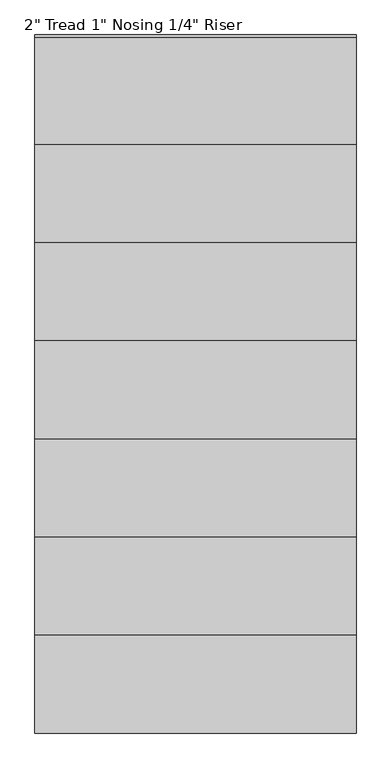
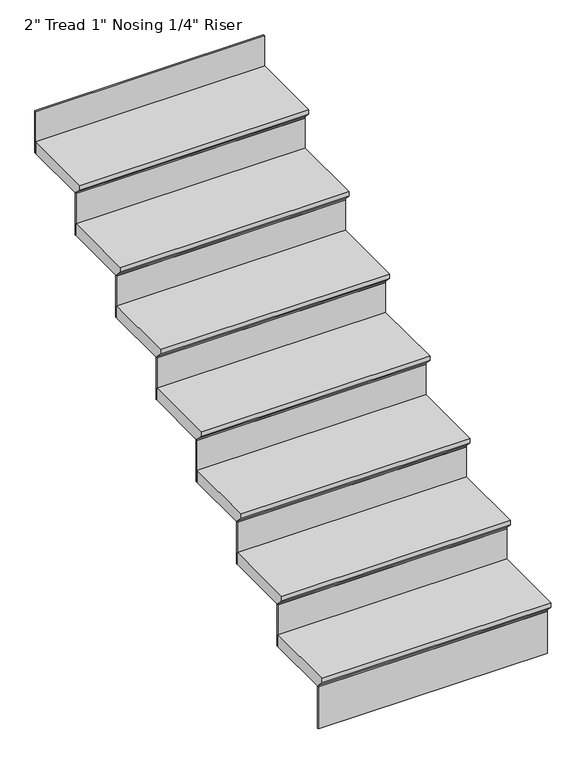
"""IFC4 building model written with IfcOpenShell, lengths in millimetres: stair flight geometry."""

from ifc_helpers import new_model, si_unit, frame, origin, place, context, project, spatial, polyline, outline, extrude, source, transform, mapped, element, save


def stair_flight_4d250dde(model_context):
    return source(origin(), model_context, "Body", "SweptSolid", [
        extrude(outline(polyline([(-3538.5064015, 5765.8), (-3233.7064015, 5765.8), (-3233.7064015, 5715.0), (-3513.1064015, 5715.0), (-3513.1064015, 5721.35), (-3538.5064015, 5746.75), (-3538.5064015, 5765.8)])), frame((-4591.1993763, 0.0, 0.0), z_axis=(1.0, 0.0, 0.0), x_axis=(0.0, 1.0, 0.0)), (0.0, 0.0, 1.0), 914.4),
        extrude(outline(polyline([(-3676.7993763, -3506.7564015), (-3676.7993763, -3513.1064015), (-4591.1993763, -3513.1064015), (-4591.1993763, -3506.7564015), (-3676.7993763, -3506.7564015)])), frame((0.0, 0.0, 5537.2), z_axis=(0.0, 0.0, 1.0), x_axis=(1.0, 0.0, 0.0)), (0.0, 0.0, 1.0), 177.8),
        extrude(outline(polyline([(-3676.7993763, -3227.3564015), (-3676.7993763, -3233.7064015), (-4591.1993763, -3233.7064015), (-4591.1993763, -3227.3564015), (-3676.7993763, -3227.3564015)])), frame((0.0, 0.0, 5715.0), z_axis=(0.0, 0.0, 1.0), x_axis=(1.0, 0.0, 0.0)), (0.0, 0.0, 1.0), 177.8),
        extrude(outline(polyline([(-3259.1064015, 5943.6), (-2954.3064015, 5943.6), (-2954.3064015, 5892.8), (-3233.7064015, 5892.8), (-3233.7064015, 5899.15), (-3259.1064015, 5924.55), (-3259.1064015, 5943.6)])), frame((-4591.1993763, 0.0, 0.0), z_axis=(1.0, 0.0, 0.0), x_axis=(0.0, 1.0, 0.0)), (0.0, 0.0, 1.0), 914.4),
        extrude(outline(polyline([(-3676.7993763, -2947.9564015), (-3676.7993763, -2954.3064015), (-4591.1993763, -2954.3064015), (-4591.1993763, -2947.9564015), (-3676.7993763, -2947.9564015)])), frame((0.0, 0.0, 5892.8), z_axis=(0.0, 0.0, 1.0), x_axis=(1.0, 0.0, 0.0)), (0.0, 0.0, 1.0), 177.8),
        extrude(outline(polyline([(-2979.7064015, 6121.4), (-2674.9064015, 6121.4), (-2674.9064015, 6070.6), (-2954.3064015, 6070.6), (-2954.3064015, 6076.95), (-2979.7064015, 6102.35), (-2979.7064015, 6121.4)])), frame((-4591.1993763, 0.0, 0.0), z_axis=(1.0, 0.0, 0.0), x_axis=(0.0, 1.0, 0.0)), (0.0, 0.0, 1.0), 914.4),
        extrude(outline(polyline([(-3676.7993763, -2668.5564015), (-3676.7993763, -2674.9064015), (-4591.1993763, -2674.9064015), (-4591.1993763, -2668.5564015), (-3676.7993763, -2668.5564015)])), frame((0.0, 0.0, 6070.6), z_axis=(0.0, 0.0, 1.0), x_axis=(1.0, 0.0, 0.0)), (0.0, 0.0, 1.0), 177.8),
        extrude(outline(polyline([(-2700.3064015, 6299.2), (-2395.5064015, 6299.2), (-2395.5064015, 6248.4), (-2674.9064015, 6248.4), (-2674.9064015, 6254.75), (-2700.3064015, 6280.15), (-2700.3064015, 6299.2)])), frame((-4591.1993763, 0.0, 0.0), z_axis=(1.0, 0.0, 0.0), x_axis=(0.0, 1.0, 0.0)), (0.0, 0.0, 1.0), 914.4),
        extrude(outline(polyline([(-3676.7993763, -2389.1564015), (-3676.7993763, -2395.5064015), (-4591.1993763, -2395.5064015), (-4591.1993763, -2389.1564015), (-3676.7993763, -2389.1564015)])), frame((0.0, 0.0, 6248.4), z_axis=(0.0, 0.0, 1.0), x_axis=(1.0, 0.0, 0.0)), (0.0, 0.0, 1.0), 177.8),
        extrude(outline(polyline([(-2420.9064015, 6477.0), (-2116.1064015, 6477.0), (-2116.1064015, 6426.2), (-2395.5064015, 6426.2), (-2395.5064015, 6432.55), (-2420.9064015, 6457.95), (-2420.9064015, 6477.0)])), frame((-4591.1993763, 0.0, 0.0), z_axis=(1.0, 0.0, 0.0), x_axis=(0.0, 1.0, 0.0)), (0.0, 0.0, 1.0), 914.4),
        extrude(outline(polyline([(-3676.7993763, -2109.7564015), (-3676.7993763, -2116.1064015), (-4591.1993763, -2116.1064015), (-4591.1993763, -2109.7564015), (-3676.7993763, -2109.7564015)])), frame((0.0, 0.0, 6426.2), z_axis=(0.0, 0.0, 1.0), x_axis=(1.0, 0.0, 0.0)), (0.0, 0.0, 1.0), 177.8),
        extrude(outline(polyline([(-2141.5064015, 6654.8), (-1836.7064015, 6654.8), (-1836.7064015, 6604.0), (-2116.1064015, 6604.0), (-2116.1064015, 6610.35), (-2141.5064015, 6635.75), (-2141.5064015, 6654.8)])), frame((-4591.1993763, 0.0, 0.0), z_axis=(1.0, 0.0, 0.0), x_axis=(0.0, 1.0, 0.0)), (0.0, 0.0, 1.0), 914.4),
        extrude(outline(polyline([(-3676.7993763, -1830.3564015), (-3676.7993763, -1836.7064015), (-4591.1993763, -1836.7064015), (-4591.1993763, -1830.3564015), (-3676.7993763, -1830.3564015)])), frame((0.0, 0.0, 6604.0), z_axis=(0.0, 0.0, 1.0), x_axis=(1.0, 0.0, 0.0)), (0.0, 0.0, 1.0), 177.8),
        extrude(outline(polyline([(-3676.7993763, -1550.9564015), (-3676.7993763, -1557.3064015), (-4591.1993763, -1557.3064015), (-4591.1993763, -1550.9564015), (-3676.7993763, -1550.9564015)])), frame((0.0, 0.0, 6781.8), z_axis=(0.0, 0.0, 1.0), x_axis=(1.0, 0.0, 0.0)), (0.0, 0.0, 1.0), 177.8),
        extrude(outline(polyline([(-1862.1064015, 6832.6), (-1557.3064015, 6832.6), (-1557.3064015, 6781.8), (-1836.7064015, 6781.8), (-1836.7064015, 6788.15), (-1862.1064015, 6813.55), (-1862.1064015, 6832.6)])), frame((-4591.1993763, 0.0, 0.0), z_axis=(1.0, 0.0, 0.0), x_axis=(0.0, 1.0, 0.0)), (0.0, 0.0, 1.0), 914.4),
    ])


if __name__ == "__main__":
    model = new_model("IFC4")
    model_context = context("Model", 3, world=origin())
    ifc_project = project(units=[si_unit("LENGTHUNIT", "METRE", prefix="MILLI")], contexts=[model_context])
    site = spatial("IfcSite", under=ifc_project)
    building = spatial("IfcBuilding", under=site)
    placement = place(None, origin())
    stair_flight_shape = stair_flight_4d250dde(model_context)
    element("IfcStairFlight", 1, ObjectType="2\" Tread 1\" Nosing 1/4\" Riser", at=placement, inside=building, context=model_context, shape_type="MappedRepresentation", body=[
        mapped(stair_flight_shape, transform((0.0, 0.0, 0.0), x_axis=(1.0, 0.0, 0.0), y_axis=(0.0, 1.0, 0.0), z_axis=(0.0, 0.0, 1.0))),
    ])
    save(model, "model.ifc")
